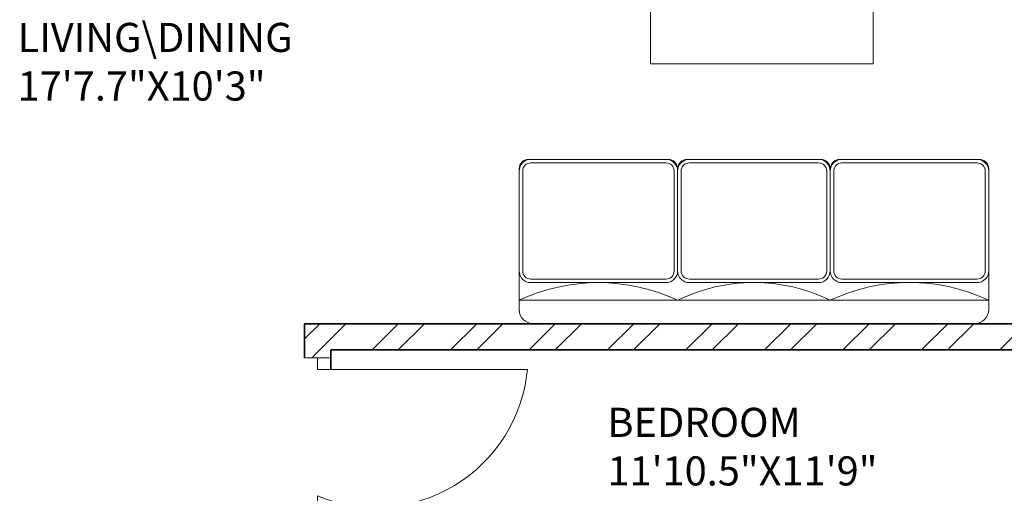
# Model space of a CAD drawing. Units: inches. Extents: x 2120 to 4013, y 1390 to 3019.
# Tile 12 of 59: x 2448 to 2617, y 1702 to 1784. Entities that reach past the tile are written whole.
import ezdxf

# ---------------------------------------------------------------- set-up
doc = ezdxf.new("R2010")
doc.units = ezdxf.units.IN
for name, color, linetype, lineweight in [('A-AREA-IDEN', 7, 'Continuous', 18), ('A-DOOR', 3, 'Continuous', 18), ('A-FURN', 8, 'Continuous', 13), ('A-WALL', 7, 'Continuous', 35), ('A-WALL-PATT', 252, 'Continuous', 13)]:
    doc.layers.add(name, color=color, linetype=linetype, lineweight=lineweight)
doc.styles.get("Standard").update_dxf_attribs({"font": 'arial.ttf'})

# ---------------------------------------------------------------- blocks, each defined once
blk = doc.blocks.new('DOOR-SWING-36IN-107p00DEG')
for p, q in [((4.5, 26.58), (0, 26.58)), ((0, 26.58), (2.25, 26.58)), ((2.25, 26.58), (2.25, 24.58)), ((2.25, 24.58), (38.25, 24.58)), ((2.25, 0), (2.25, 2.87)), ((4.5, 0), (0, 0)), ((0, 0), (2.25, 0))]:
    blk.add_line(p, q)
blk.add_arc((12.22, 27.04), 26.15, 247.599, 354.5999)
blk = doc.blocks.new('TABLE-COFFEE')
blk.add_lwpolyline([(0, 38.19), (21.88, 38.19), (21.88, 0), (0, 0)], close=True)

msp = doc.modelspace()

# ---------------------------------------------------------------- hatches: boundary and pattern name
at = {"layer": 'A-WALL-PATT'}
h = msp.add_hatch(dxfattribs=at)
h.set_pattern_fill('ANSI32', color=256)
h.paths.add_polyline_path([(2271.7331, 2343.531), (2283.3788, 2343.531), (2283.3788, 2348.031), (2283.3788, 2352.5306), (2262.7331, 2352.5306), (2262.7331, 2182.638), (2267.2331, 2182.638), (2271.7331, 2182.638), (2271.7331, 2219.031), (2391.7331, 2219.031), (2391.7331, 2214.189), (2393.9831, 2214.189), (2396.2331, 2214.189), (2396.2331, 2219.031), (2420.2331, 2219.031), (2420.2331, 2225.7535), (2417.2197, 2225.7535), (2415.7331, 2225.7535), (2415.7331, 2223.5306), (2271.7331, 2223.5306)])
h.paths.add_polyline_path([(2380.0942, 2352.5306), (2343.3788, 2352.5306), (2343.3788, 2343.531), (2363.2331, 2343.531), (2363.2331, 2288.8489), (2365.4831, 2288.8489), (2367.7331, 2288.8489), (2367.7331, 2343.531), (2380.0942, 2343.531)], flags=17)
h.paths.add_polyline_path([(2432.4339, 2352.5306), (2404.0943, 2352.5306), (2404.0943, 2343.531), (2415.7331, 2343.531), (2415.7331, 2264.0306), (2367.7331, 2264.0306), (2367.7331, 2266.4872), (2363.2331, 2266.4872), (2363.2331, 2259.531), (2367.7331, 2259.531), (2415.7331, 2259.531), (2415.7331, 2255.0658), (2420.2331, 2255.0658), (2420.2331, 2259.531), (2424.5717, 2259.531), (2424.5717, 2261.781), (2424.5717, 2264.0306), (2420.2331, 2264.0306), (2420.2331, 2343.531), (2432.4339, 2343.531)])
h.paths.add_polyline_path([(2508.9115, 2352.5306), (2456.4339, 2352.5306), (2456.4339, 2343.531), (2468.2331, 2343.531), (2468.2331, 2264.0306), (2448.0487, 2264.0306), (2448.0487, 2259.531), (2468.2331, 2259.531), (2468.2331, 2255.5496), (2472.7331, 2255.5496), (2472.7331, 2343.531), (2508.9115, 2343.531)])
h.paths.add_polyline_path([(2637.7331, 2352.5306), (2544.9116, 2352.5306), (2544.9116, 2343.531), (2589.7331, 2343.531), (2633.2331, 2343.531), (2637.7331, 2343.531)])
h.paths.add_polyline_path([(2594.2331, 2343.5306), (2589.7331, 2343.5306), (2589.7331, 2259.5306), (2589.7331, 2252.4915), (2591.9831, 2252.4915), (2594.2331, 2252.4915)])
h.paths.add_polyline_path([(2637.7331, 2223.5306), (2594.2331, 2223.5306), (2594.2331, 2230.1988), (2591.9831, 2230.1988), (2589.7331, 2230.1988), (2589.7331, 2223.5306), (2472.7331, 2223.5306), (2468.2331, 2223.5306), (2468.2331, 2219.031), (2628.7331, 2219.031), (2628.7331, 2138.031), (2637.7331, 2138.031)])
h.paths.add_polyline_path([(3822.6535, 2458.4402), (3874.9468, 2458.4402), (3874.9468, 2476.9866), (3822.6535, 2476.9866)], flags=9)
h.paths.add_polyline_path([(3834.6921, 2781.8174), (3935.9206, 2781.8174), (3935.9206, 2800.3638), (3834.6921, 2800.3638)], flags=9)
h.paths.add_polyline_path([(3832.2843, 2837.9683), (3884.5776, 2837.9683), (3884.5776, 2856.5146), (3832.2843, 2856.5146)], flags=9)
h.paths.add_polyline_path([(3830.9388, 2861.4782), (3956.8958, 2861.4782), (3956.8958, 2880.0245), (3830.9388, 2880.0245)], flags=9)
h.paths.add_polyline_path([(3870.6966, 2352.5752), (3887.9272, 2352.5752), (3887.9272, 2377.3037), (3870.6966, 2377.3037)], flags=9)
h.paths.add_polyline_path([(3289.2701, 2413.161), (3435.2223, 2413.161), (3435.2223, 2450.2538), (3289.2701, 2450.2538)], flags=9)
h.paths.add_polyline_path([(2487.6944, 2414.3601), (2637.8335, 2414.3601), (2637.8335, 2451.4528), (2487.6944, 2451.4528)], flags=9)
h.paths.add_polyline_path([(2567.3724, 1457.9199), (2815.296, 1457.9199), (2815.296, 1495.0127), (2567.3724, 1495.0127)], flags=9)
h.paths.add_polyline_path([(2655.3825, 2093.2363), (2685.9555, 2093.2363), (2685.9555, 2111.8937), (2655.3825, 2111.8937)], flags=9)
h.paths.add_polyline_path([(2543.9218, 1550.6671), (2587.8406, 1550.6671), (2587.8406, 1569.3244), (2543.9218, 1569.3244)], flags=9)
h.paths.add_polyline_path([(2905.1384, 1543.8113), (2949.0572, 1543.8113), (2949.0572, 1562.4686), (2905.1384, 1562.4686)], flags=9)
h.paths.add_polyline_path([(2736.4118, 1702.4736), (2784.2153, 1702.4736), (2784.2153, 1721.1309), (2736.4118, 1721.1309)], flags=9)
h.paths.add_polyline_path([(2912.8666, 1710.4168), (2951.707, 1710.4168), (2951.707, 1729.0741), (2912.8666, 1729.0741)], flags=9)
h.paths.add_polyline_path([(2923.5785, 1763.5038), (2959.7279, 1763.5038), (2959.7279, 1782.1611), (2923.5785, 1782.1611)], flags=9)
h.paths.add_polyline_path([(2925.2114, 1809.6137), (2967.1861, 1809.6137), (2967.1861, 1828.271), (2925.2114, 1828.271)], flags=9)
h.paths.add_polyline_path([(2996.2711, 1878.9003), (2996.2711, 1913.109), (2977.6138, 1913.109), (2977.6138, 1878.9003)], flags=9)
h.paths.add_polyline_path([(2883.0859, 1895.7192), (2927.1855, 1895.7192), (2927.1855, 1914.3766), (2883.0859, 1914.3766)], flags=9)
h.paths.add_polyline_path([(2787.3924, 1810.8013), (2841.0213, 1810.8013), (2841.0213, 1829.4587), (2787.3924, 1829.4587)], flags=9)
h.paths.add_polyline_path([(2775.6399, 2101.7395), (2829.2689, 2101.7395), (2829.2689, 2120.3968), (2775.6399, 2120.3968)], flags=9)
h.paths.add_polyline_path([(2913.0263, 2075.817), (2951.8667, 2075.817), (2951.8667, 2094.4744), (2913.0263, 2094.4744)], flags=9)
h.paths.add_polyline_path([(2929.966, 2133.3669), (2966.1154, 2133.3669), (2966.1154, 2152.0243), (2929.966, 2152.0243)], flags=9)
h.paths.add_polyline_path([(2932.7502, 2182.6088), (2968.8996, 2182.6088), (2968.8996, 2201.2662), (2932.7502, 2201.2662)], flags=9)
h.paths.add_polyline_path([(2996.0681, 2266.3173), (2996.0681, 2300.5261), (2977.4108, 2300.5261), (2977.4108, 2266.3173)], flags=9)
h.paths.add_polyline_path([(2885.1039, 2279.2186), (2929.2035, 2279.2186), (2929.2035, 2297.8759), (2885.1039, 2297.8759)], flags=9)
h.paths.add_polyline_path([(2735.7042, 2218.3197), (2783.5078, 2218.3197), (2783.5078, 2236.9771), (2735.7042, 2236.9771)], flags=9)
h.paths.add_polyline_path([(2635.6049, 2044.0085), (2648.9678, 2044.0085), (2648.9678, 2054.312), (2635.6049, 2054.312)], flags=9)
h.paths.add_polyline_path([(2714.0148, 1923.0473), (2727.3777, 1923.0473), (2727.3777, 1933.3508), (2714.0148, 1933.3508)], flags=9)
h.paths.add_polyline_path([(2709.0345, 1988.1628), (2722.3974, 1988.1628), (2722.3974, 1998.4663), (2709.0345, 1998.4663)], flags=9)
h.paths.add_polyline_path([(2592.8935, 1962.1763), (2606.2564, 1962.1763), (2606.2564, 1972.4799), (2592.8935, 1972.4799)], flags=9)
h.paths.add_polyline_path([(2618.3996, 1985.9724), (2644.1942, 1985.9724), (2644.1942, 1996.2759), (2618.3996, 1996.2759)], flags=9)
h.paths.add_polyline_path([(2601.279, 1920.5869), (2614.6419, 1920.5869), (2614.6419, 1930.8904), (2601.279, 1930.8904)], flags=9)
h.paths.add_polyline_path([(2692.3278, 1932.7645), (2704.5311, 1932.7645), (2704.5311, 1943.0681), (2692.3278, 1943.0681)], flags=9)
h.paths.add_polyline_path([(2311.122, 1672.7318), (2355.0408, 1672.7318), (2355.0408, 1691.3892), (2311.122, 1691.3892)], flags=9)
h.paths.add_polyline_path([(2456.2551, 1632.3198), (2492.4796, 1632.3198), (2492.4796, 1650.9772), (2456.2551, 1650.9772)], flags=9)
h.paths.add_polyline_path([(2401.0766, 1631.4793), (2437.301, 1631.4793), (2437.301, 1650.1367), (2401.0766, 1650.1367)], flags=9)
h.paths.add_polyline_path([(2546.7054, 1700.9235), (2594.509, 1700.9235), (2594.509, 1719.5809), (2546.7054, 1719.5809)], flags=9)
h.paths.add_polyline_path([(2445.4866, 1766.9937), (2497.5261, 1766.9937), (2497.5261, 1785.651), (2445.4866, 1785.651)], flags=9)
h.paths.add_polyline_path([(2287.9992, 1739.7675), (2326.8396, 1739.7675), (2326.8396, 1758.4248), (2287.9992, 1758.4248)], flags=9)
h.paths.add_polyline_path([(2458.5279, 1924.7607), (2510.5675, 1924.7607), (2510.5675, 1943.4181), (2458.5279, 1943.4181)], flags=9)
h.paths.add_polyline_path([(2309.2811, 1902.7642), (2345.4305, 1902.7642), (2345.4305, 1921.4215), (2309.2811, 1921.4215)], flags=9)
h.paths.add_polyline_path([(2490.7554, 2018.9392), (2530.7896, 2018.9392), (2530.7896, 2037.5965), (2490.7554, 2037.5965)], flags=9)
h.paths.add_polyline_path([(2402.143, 2024.7393), (2438.5414, 2024.7393), (2438.5414, 2043.3966), (2402.143, 2043.3966)], flags=9)
h.paths.add_polyline_path([(2287.856, 1931.7926), (2326.6964, 1931.7926), (2326.6964, 1950.4499), (2287.856, 1950.4499)], flags=9)
h.paths.add_polyline_path([(2281.7979, 2193.5771), (2320.6383, 2193.5771), (2320.6383, 2212.2344), (2281.7979, 2212.2344)], flags=25)
h.paths.add_polyline_path([(2484.0754, 2093.892), (2536.115, 2093.892), (2536.115, 2112.5494), (2484.0754, 2112.5494)], flags=9)
h.paths.add_polyline_path([(2624.7948, 2281.8639), (2624.7948, 2311.4137), (2606.1375, 2311.4137), (2606.1375, 2281.8639)], flags=9)
h.paths.add_polyline_path([(2507.5036, 2290.3639), (2541.934, 2290.3639), (2541.934, 2309.0212), (2507.5036, 2309.0212)], flags=9)
h.paths.add_polyline_path([(2423.1076, 2285.2202), (2459.332, 2285.2202), (2459.332, 2303.8776), (2423.1076, 2303.8776)], flags=9)
h.paths.add_polyline_path([(2374.5467, 2289.6272), (2410.7711, 2289.6272), (2410.7711, 2308.2846), (2374.5467, 2308.2846)], flags=25)
h.paths.add_polyline_path([(2277.4907, 2227.5651), (2316.3311, 2227.5651), (2316.3311, 2246.2224), (2277.4907, 2246.2224)], flags=25)
h.paths.add_polyline_path([(2655.3825, 2093.2367), (2685.9555, 2093.2367), (2685.9555, 2111.894), (2655.3825, 2111.894)], flags=9)
h.paths.add_polyline_path([(2543.9217, 1550.6674), (2587.8406, 1550.6674), (2587.8406, 1569.3247), (2543.9217, 1569.3247)], flags=9)
h.paths.add_polyline_path([(2905.1384, 1543.8116), (2949.0572, 1543.8116), (2949.0572, 1562.4689), (2905.1384, 1562.4689)], flags=9)
h.paths.add_polyline_path([(2736.4118, 1702.4739), (2784.2153, 1702.4739), (2784.2153, 1721.1312), (2736.4118, 1721.1312)], flags=9)
h.paths.add_polyline_path([(2912.8666, 1710.4171), (2951.707, 1710.4171), (2951.707, 1729.0744), (2912.8666, 1729.0744)], flags=9)
h.paths.add_polyline_path([(2923.5785, 1763.5041), (2959.7279, 1763.5041), (2959.7279, 1782.1614), (2923.5785, 1782.1614)], flags=9)
h.paths.add_polyline_path([(2925.2114, 1809.614), (2967.1861, 1809.614), (2967.1861, 1828.2713), (2925.2114, 1828.2713)], flags=9)
h.paths.add_polyline_path([(2996.2711, 1878.9006), (2996.2711, 1913.1094), (2977.6137, 1913.1094), (2977.6137, 1878.9006)], flags=9)
h.paths.add_polyline_path([(2883.0859, 1895.7195), (2927.1855, 1895.7195), (2927.1855, 1914.3769), (2883.0859, 1914.3769)], flags=9)
h.paths.add_polyline_path([(2787.3924, 1810.8016), (2841.0213, 1810.8016), (2841.0213, 1829.459), (2787.3924, 1829.459)], flags=9)
h.paths.add_polyline_path([(2775.6399, 2101.7398), (2829.2688, 2101.7398), (2829.2688, 2120.3971), (2775.6399, 2120.3971)], flags=9)
h.paths.add_polyline_path([(2913.0263, 2075.8173), (2951.8667, 2075.8173), (2951.8667, 2094.4747), (2913.0263, 2094.4747)], flags=9)
h.paths.add_polyline_path([(2929.966, 2133.3672), (2966.1154, 2133.3672), (2966.1154, 2152.0246), (2929.966, 2152.0246)], flags=9)
h.paths.add_polyline_path([(2932.7502, 2182.6091), (2968.8996, 2182.6091), (2968.8996, 2201.2665), (2932.7502, 2201.2665)], flags=9)
h.paths.add_polyline_path([(2996.0681, 2266.3176), (2996.0681, 2300.5264), (2977.4108, 2300.5264), (2977.4108, 2266.3176)], flags=9)
h.paths.add_polyline_path([(2885.1039, 2279.2189), (2929.2035, 2279.2189), (2929.2035, 2297.8762), (2885.1039, 2297.8762)], flags=9)
h.paths.add_polyline_path([(2735.7042, 2218.32), (2783.5078, 2218.32), (2783.5078, 2236.9774), (2735.7042, 2236.9774)], flags=9)
h.paths.add_polyline_path([(2635.6048, 2044.0088), (2648.9677, 2044.0088), (2648.9677, 2054.3123), (2635.6048, 2054.3123)], flags=9)
h.paths.add_polyline_path([(2714.0148, 1923.0476), (2727.3777, 1923.0476), (2727.3777, 1933.3511), (2714.0148, 1933.3511)], flags=9)
h.paths.add_polyline_path([(2709.0345, 1988.1631), (2722.3974, 1988.1631), (2722.3974, 1998.4666), (2709.0345, 1998.4666)], flags=9)
h.paths.add_polyline_path([(2592.8935, 1962.1766), (2606.2564, 1962.1766), (2606.2564, 1972.4802), (2592.8935, 1972.4802)], flags=9)
h.paths.add_polyline_path([(2618.3995, 1985.9727), (2644.1942, 1985.9727), (2644.1942, 1996.2762), (2618.3995, 1996.2762)], flags=9)
h.paths.add_polyline_path([(2601.279, 1920.5872), (2614.6419, 1920.5872), (2614.6419, 1930.8908), (2601.279, 1930.8908)], flags=9)
h.paths.add_polyline_path([(2692.3278, 1932.7648), (2704.5311, 1932.7648), (2704.5311, 1943.0684), (2692.3278, 1943.0684)], flags=9)
h.paths.add_polyline_path([(2311.122, 1672.7321), (2355.0408, 1672.7321), (2355.0408, 1691.3895), (2311.122, 1691.3895)], flags=9)
h.paths.add_polyline_path([(2456.2551, 1632.3201), (2492.4795, 1632.3201), (2492.4795, 1650.9775), (2456.2551, 1650.9775)], flags=9)
h.paths.add_polyline_path([(2401.0766, 1631.4796), (2437.301, 1631.4796), (2437.301, 1650.137), (2401.0766, 1650.137)], flags=9)
h.paths.add_polyline_path([(2546.7054, 1700.9238), (2594.509, 1700.9238), (2594.509, 1719.5812), (2546.7054, 1719.5812)], flags=9)
h.paths.add_polyline_path([(2445.4866, 1766.994), (2497.5261, 1766.994), (2497.5261, 1785.6513), (2445.4866, 1785.6513)], flags=9)
h.paths.add_polyline_path([(2287.9992, 1739.7678), (2326.8396, 1739.7678), (2326.8396, 1758.4251), (2287.9992, 1758.4251)], flags=9)
h.paths.add_polyline_path([(2458.5279, 1924.7611), (2510.5675, 1924.7611), (2510.5675, 1943.4184), (2458.5279, 1943.4184)], flags=9)
h.paths.add_polyline_path([(2309.2811, 1902.7645), (2345.4305, 1902.7645), (2345.4305, 1921.4218), (2309.2811, 1921.4218)], flags=9)
h.paths.add_polyline_path([(2490.7554, 2018.9395), (2530.7895, 2018.9395), (2530.7895, 2037.5968), (2490.7554, 2037.5968)], flags=9)
h.paths.add_polyline_path([(2402.143, 2024.7396), (2438.5413, 2024.7396), (2438.5413, 2043.3969), (2402.143, 2043.3969)], flags=9)
h.paths.add_polyline_path([(2287.856, 1931.7929), (2326.6964, 1931.7929), (2326.6964, 1950.4502), (2287.856, 1950.4502)], flags=9)
h.paths.add_polyline_path([(2281.7979, 2193.5774), (2320.6383, 2193.5774), (2320.6383, 2212.2347), (2281.7979, 2212.2347)], flags=25)
h.paths.add_polyline_path([(2484.0754, 2093.8924), (2536.115, 2093.8924), (2536.115, 2112.5497), (2484.0754, 2112.5497)], flags=9)
h.paths.add_polyline_path([(2624.7948, 2281.8642), (2624.7948, 2311.414), (2606.1374, 2311.414), (2606.1374, 2281.8642)], flags=9)
h.paths.add_polyline_path([(2507.5035, 2290.3642), (2541.934, 2290.3642), (2541.934, 2309.0215), (2507.5035, 2309.0215)], flags=9)
h.paths.add_polyline_path([(2423.1075, 2285.2205), (2459.332, 2285.2205), (2459.332, 2303.8779), (2423.1075, 2303.8779)], flags=9)
h.paths.add_polyline_path([(2374.5467, 2289.6275), (2410.7711, 2289.6275), (2410.7711, 2308.2849), (2374.5467, 2308.2849)], flags=25)
h.paths.add_polyline_path([(2277.4907, 2227.5654), (2316.3311, 2227.5654), (2316.3311, 2246.2227), (2277.4907, 2246.2227)], flags=25)
h = msp.add_hatch(dxfattribs=at)
h.set_pattern_fill('ANSI32', color=256)
h.paths.add_polyline_path([(2271.7331, 1980.389), (2262.7331, 1980.389), (2262.7331, 1912.8434), (2267.2331, 1912.8434), (2271.7331, 1912.8434), (2271.7331, 1922.531), (2351.2331, 1922.531), (2351.2331, 1901.4728), (2355.7331, 1901.4728), (2355.7331, 1922.531), (2357.9815, 1922.531), (2357.9815, 1926.5306), (2271.7331, 1926.5306)])
h.paths.add_polyline_path([(2589.2331, 1949.1622), (2584.7331, 1949.1622), (2580.2331, 1949.1622), (2580.2331, 1874.5306), (2355.7331, 1874.5306), (2355.7331, 1880.1922), (2351.2331, 1880.1922), (2351.2331, 1874.5306), (2271.7331, 1874.5306), (2271.7331, 1888.8431), (2262.7331, 1888.8431), (2262.7331, 1842.2909), (2267.2331, 1842.2909), (2271.7331, 1842.2909), (2271.7331, 1865.531), (2415.7331, 1865.531), (2415.7331, 1779.7286), (2420.2331, 1779.7286), (2420.2331, 1865.531), (2589.2331, 1865.531)])
h.paths.add_polyline_path([(2271.7331, 1782.2906), (2262.7331, 1782.2906), (2262.7331, 1711.4639), (2267.2331, 1711.4639), (2271.7331, 1711.4639), (2271.7331, 1738.031), (2420.2331, 1738.031), (2420.2331, 1742.531), (2420.2331, 1747.3376), (2417.9831, 1747.3376), (2415.7331, 1747.3376), (2415.7331, 1742.5306), (2271.7331, 1742.5306)])
h.paths.add_polyline_path([(2271.7331, 1627.031), (2362.3957, 1627.031), (2362.3957, 1629.281), (2362.3957, 1631.5306), (2271.7331, 1631.5306), (2271.7331, 1675.4636), (2262.7331, 1675.4636), (2262.7331, 1581.531), (2405.3032, 1581.531), (2405.3032, 1586.031), (2405.3032, 1590.5306), (2396.2331, 1590.5306), (2396.2331, 1691.4513), (2418.7206, 1691.4513), (2418.7206, 1695.951), (2396.2331, 1695.951), (2391.7331, 1695.951), (2391.7331, 1631.5306), (2386.7425, 1631.5306), (2386.7425, 1629.2806), (2386.7425, 1627.031), (2391.7331, 1627.031), (2391.7331, 1586.1709), (2271.7331, 1586.1709)])
h.paths.add_polyline_path([(2459.6703, 1590.5306), (2429.3032, 1590.5306), (2429.3032, 1581.531), (2459.6703, 1581.531), (2459.6703, 1586.031)])
h.paths.add_polyline_path([(2501.2331, 1590.531), (2501.2331, 1665.0195), (2498.9831, 1665.0195), (2496.7331, 1665.0195), (2496.7331, 1590.5306), (2483.8201, 1590.5306), (2483.8201, 1590.1579), (2483.6704, 1590.1579), (2483.6704, 1581.531), (2505.0196, 1581.531), (2505.0196, 1583.781), (2505.0196, 1586.0306), (2501.2331, 1586.0306)])
h.paths.add_polyline_path([(2544.1361, 1583.781), (2544.1361, 1586.0306), (2527.1368, 1586.0306), (2527.1368, 1583.7806), (2527.1368, 1581.531), (2544.1361, 1581.531)])
h.paths.add_polyline_path([(3822.6535, 2458.4402), (3874.9468, 2458.4402), (3874.9468, 2476.9866), (3822.6535, 2476.9866)], flags=9)
h.paths.add_polyline_path([(3834.6921, 2781.8174), (3935.9206, 2781.8174), (3935.9206, 2800.3638), (3834.6921, 2800.3638)], flags=9)
h.paths.add_polyline_path([(3832.2843, 2837.9683), (3884.5776, 2837.9683), (3884.5776, 2856.5146), (3832.2843, 2856.5146)], flags=9)
h.paths.add_polyline_path([(3830.9388, 2861.4782), (3956.8958, 2861.4782), (3956.8958, 2880.0245), (3830.9388, 2880.0245)], flags=9)
h.paths.add_polyline_path([(3870.6966, 2352.5752), (3887.9272, 2352.5752), (3887.9272, 2377.3037), (3870.6966, 2377.3037)], flags=9)
h.paths.add_polyline_path([(3289.2701, 2413.161), (3435.2223, 2413.161), (3435.2223, 2450.2538), (3289.2701, 2450.2538)], flags=9)
h.paths.add_polyline_path([(2487.6944, 2414.3601), (2637.8335, 2414.3601), (2637.8335, 2451.4528), (2487.6944, 2451.4528)], flags=9)
h.paths.add_polyline_path([(2567.3724, 1457.9199), (2815.296, 1457.9199), (2815.296, 1495.0127), (2567.3724, 1495.0127)], flags=9)
h.paths.add_polyline_path([(2655.3825, 2093.2363), (2685.9555, 2093.2363), (2685.9555, 2111.8937), (2655.3825, 2111.8937)], flags=9)
h.paths.add_polyline_path([(2543.9218, 1550.6671), (2587.8406, 1550.6671), (2587.8406, 1569.3244), (2543.9218, 1569.3244)], flags=9)
h.paths.add_polyline_path([(2905.1384, 1543.8113), (2949.0572, 1543.8113), (2949.0572, 1562.4686), (2905.1384, 1562.4686)], flags=9)
h.paths.add_polyline_path([(2736.4118, 1702.4736), (2784.2153, 1702.4736), (2784.2153, 1721.1309), (2736.4118, 1721.1309)], flags=9)
h.paths.add_polyline_path([(2912.8666, 1710.4168), (2951.707, 1710.4168), (2951.707, 1729.0741), (2912.8666, 1729.0741)], flags=9)
h.paths.add_polyline_path([(2923.5785, 1763.5038), (2959.7279, 1763.5038), (2959.7279, 1782.1611), (2923.5785, 1782.1611)], flags=9)
h.paths.add_polyline_path([(2925.2114, 1809.6137), (2967.1861, 1809.6137), (2967.1861, 1828.271), (2925.2114, 1828.271)], flags=9)
h.paths.add_polyline_path([(2996.2711, 1878.9003), (2996.2711, 1913.109), (2977.6138, 1913.109), (2977.6138, 1878.9003)], flags=9)
h.paths.add_polyline_path([(2883.0859, 1895.7192), (2927.1855, 1895.7192), (2927.1855, 1914.3766), (2883.0859, 1914.3766)], flags=9)
h.paths.add_polyline_path([(2787.3924, 1810.8013), (2841.0213, 1810.8013), (2841.0213, 1829.4587), (2787.3924, 1829.4587)], flags=9)
h.paths.add_polyline_path([(2775.6399, 2101.7395), (2829.2689, 2101.7395), (2829.2689, 2120.3968), (2775.6399, 2120.3968)], flags=9)
h.paths.add_polyline_path([(2913.0263, 2075.817), (2951.8667, 2075.817), (2951.8667, 2094.4744), (2913.0263, 2094.4744)], flags=9)
h.paths.add_polyline_path([(2929.966, 2133.3669), (2966.1154, 2133.3669), (2966.1154, 2152.0243), (2929.966, 2152.0243)], flags=9)
h.paths.add_polyline_path([(2932.7502, 2182.6088), (2968.8996, 2182.6088), (2968.8996, 2201.2662), (2932.7502, 2201.2662)], flags=9)
h.paths.add_polyline_path([(2996.0681, 2266.3173), (2996.0681, 2300.5261), (2977.4108, 2300.5261), (2977.4108, 2266.3173)], flags=9)
h.paths.add_polyline_path([(2885.1039, 2279.2186), (2929.2035, 2279.2186), (2929.2035, 2297.8759), (2885.1039, 2297.8759)], flags=9)
h.paths.add_polyline_path([(2735.7042, 2218.3197), (2783.5078, 2218.3197), (2783.5078, 2236.9771), (2735.7042, 2236.9771)], flags=9)
h.paths.add_polyline_path([(2635.6049, 2044.0085), (2648.9678, 2044.0085), (2648.9678, 2054.312), (2635.6049, 2054.312)], flags=9)
h.paths.add_polyline_path([(2714.0148, 1923.0473), (2727.3777, 1923.0473), (2727.3777, 1933.3508), (2714.0148, 1933.3508)], flags=9)
h.paths.add_polyline_path([(2709.0345, 1988.1628), (2722.3974, 1988.1628), (2722.3974, 1998.4663), (2709.0345, 1998.4663)], flags=9)
h.paths.add_polyline_path([(2592.8935, 1962.1763), (2606.2564, 1962.1763), (2606.2564, 1972.4799), (2592.8935, 1972.4799)], flags=9)
h.paths.add_polyline_path([(2618.3996, 1985.9724), (2644.1942, 1985.9724), (2644.1942, 1996.2759), (2618.3996, 1996.2759)], flags=9)
h.paths.add_polyline_path([(2601.279, 1920.5869), (2614.6419, 1920.5869), (2614.6419, 1930.8904), (2601.279, 1930.8904)], flags=9)
h.paths.add_polyline_path([(2692.3278, 1932.7645), (2704.5311, 1932.7645), (2704.5311, 1943.0681), (2692.3278, 1943.0681)], flags=9)
h.paths.add_polyline_path([(2311.122, 1672.7318), (2355.0408, 1672.7318), (2355.0408, 1691.3892), (2311.122, 1691.3892)], flags=25)
h.paths.add_polyline_path([(2456.2551, 1632.3198), (2492.4796, 1632.3198), (2492.4796, 1650.9772), (2456.2551, 1650.9772)], flags=9)
h.paths.add_polyline_path([(2401.0766, 1631.4793), (2437.301, 1631.4793), (2437.301, 1650.1367), (2401.0766, 1650.1367)], flags=9)
h.paths.add_polyline_path([(2546.7054, 1700.9235), (2594.509, 1700.9235), (2594.509, 1719.5809), (2546.7054, 1719.5809)], flags=9)
h.paths.add_polyline_path([(2445.4866, 1766.9937), (2497.5261, 1766.9937), (2497.5261, 1785.651), (2445.4866, 1785.651)], flags=9)
h.paths.add_polyline_path([(2287.9992, 1739.7675), (2326.8396, 1739.7675), (2326.8396, 1758.4248), (2287.9992, 1758.4248)], flags=24)
h.paths.add_polyline_path([(2458.5279, 1924.7607), (2510.5675, 1924.7607), (2510.5675, 1943.4181), (2458.5279, 1943.4181)], flags=25)
h.paths.add_polyline_path([(2309.2811, 1902.7642), (2345.4305, 1902.7642), (2345.4305, 1921.4215), (2309.2811, 1921.4215)], flags=25)
h.paths.add_polyline_path([(2490.7554, 2018.9392), (2530.7896, 2018.9392), (2530.7896, 2037.5965), (2490.7554, 2037.5965)], flags=9)
h.paths.add_polyline_path([(2402.143, 2024.7393), (2438.5414, 2024.7393), (2438.5414, 2043.3966), (2402.143, 2043.3966)], flags=9)
h.paths.add_polyline_path([(2287.856, 1931.7926), (2326.6964, 1931.7926), (2326.6964, 1950.4499), (2287.856, 1950.4499)], flags=25)
h.paths.add_polyline_path([(2281.7979, 2193.5771), (2320.6383, 2193.5771), (2320.6383, 2212.2344), (2281.7979, 2212.2344)], flags=9)
h.paths.add_polyline_path([(2484.0754, 2093.892), (2536.115, 2093.892), (2536.115, 2112.5494), (2484.0754, 2112.5494)], flags=9)
h.paths.add_polyline_path([(2624.7948, 2281.8639), (2624.7948, 2311.4137), (2606.1375, 2311.4137), (2606.1375, 2281.8639)], flags=9)
h.paths.add_polyline_path([(2507.5036, 2290.3639), (2541.934, 2290.3639), (2541.934, 2309.0212), (2507.5036, 2309.0212)], flags=9)
h.paths.add_polyline_path([(2423.1076, 2285.2202), (2459.332, 2285.2202), (2459.332, 2303.8776), (2423.1076, 2303.8776)], flags=9)
h.paths.add_polyline_path([(2374.5467, 2289.6272), (2410.7711, 2289.6272), (2410.7711, 2308.2846), (2374.5467, 2308.2846)], flags=9)
h.paths.add_polyline_path([(2277.4907, 2227.5651), (2316.3311, 2227.5651), (2316.3311, 2246.2224), (2277.4907, 2246.2224)], flags=9)
h.paths.add_polyline_path([(2655.3825, 2093.2367), (2685.9555, 2093.2367), (2685.9555, 2111.894), (2655.3825, 2111.894)], flags=9)
h.paths.add_polyline_path([(2543.9217, 1550.6674), (2587.8406, 1550.6674), (2587.8406, 1569.3247), (2543.9217, 1569.3247)], flags=9)
h.paths.add_polyline_path([(2905.1384, 1543.8116), (2949.0572, 1543.8116), (2949.0572, 1562.4689), (2905.1384, 1562.4689)], flags=9)
h.paths.add_polyline_path([(2736.4118, 1702.4739), (2784.2153, 1702.4739), (2784.2153, 1721.1312), (2736.4118, 1721.1312)], flags=9)
h.paths.add_polyline_path([(2912.8666, 1710.4171), (2951.707, 1710.4171), (2951.707, 1729.0744), (2912.8666, 1729.0744)], flags=9)
h.paths.add_polyline_path([(2923.5785, 1763.5041), (2959.7279, 1763.5041), (2959.7279, 1782.1614), (2923.5785, 1782.1614)], flags=9)
h.paths.add_polyline_path([(2925.2114, 1809.614), (2967.1861, 1809.614), (2967.1861, 1828.2713), (2925.2114, 1828.2713)], flags=9)
h.paths.add_polyline_path([(2996.2711, 1878.9006), (2996.2711, 1913.1094), (2977.6137, 1913.1094), (2977.6137, 1878.9006)], flags=9)
h.paths.add_polyline_path([(2883.0859, 1895.7195), (2927.1855, 1895.7195), (2927.1855, 1914.3769), (2883.0859, 1914.3769)], flags=9)
h.paths.add_polyline_path([(2787.3924, 1810.8016), (2841.0213, 1810.8016), (2841.0213, 1829.459), (2787.3924, 1829.459)], flags=9)
h.paths.add_polyline_path([(2775.6399, 2101.7398), (2829.2688, 2101.7398), (2829.2688, 2120.3971), (2775.6399, 2120.3971)], flags=9)
h.paths.add_polyline_path([(2913.0263, 2075.8173), (2951.8667, 2075.8173), (2951.8667, 2094.4747), (2913.0263, 2094.4747)], flags=9)
h.paths.add_polyline_path([(2929.966, 2133.3672), (2966.1154, 2133.3672), (2966.1154, 2152.0246), (2929.966, 2152.0246)], flags=9)
h.paths.add_polyline_path([(2932.7502, 2182.6091), (2968.8996, 2182.6091), (2968.8996, 2201.2665), (2932.7502, 2201.2665)], flags=9)
h.paths.add_polyline_path([(2996.0681, 2266.3176), (2996.0681, 2300.5264), (2977.4108, 2300.5264), (2977.4108, 2266.3176)], flags=9)
h.paths.add_polyline_path([(2885.1039, 2279.2189), (2929.2035, 2279.2189), (2929.2035, 2297.8762), (2885.1039, 2297.8762)], flags=9)
h.paths.add_polyline_path([(2735.7042, 2218.32), (2783.5078, 2218.32), (2783.5078, 2236.9774), (2735.7042, 2236.9774)], flags=9)
h.paths.add_polyline_path([(2635.6048, 2044.0088), (2648.9677, 2044.0088), (2648.9677, 2054.3123), (2635.6048, 2054.3123)], flags=9)
h.paths.add_polyline_path([(2714.0148, 1923.0476), (2727.3777, 1923.0476), (2727.3777, 1933.3511), (2714.0148, 1933.3511)], flags=9)
h.paths.add_polyline_path([(2709.0345, 1988.1631), (2722.3974, 1988.1631), (2722.3974, 1998.4666), (2709.0345, 1998.4666)], flags=9)
h.paths.add_polyline_path([(2592.8935, 1962.1766), (2606.2564, 1962.1766), (2606.2564, 1972.4802), (2592.8935, 1972.4802)], flags=9)
h.paths.add_polyline_path([(2618.3995, 1985.9727), (2644.1942, 1985.9727), (2644.1942, 1996.2762), (2618.3995, 1996.2762)], flags=9)
h.paths.add_polyline_path([(2601.279, 1920.5872), (2614.6419, 1920.5872), (2614.6419, 1930.8908), (2601.279, 1930.8908)], flags=9)
h.paths.add_polyline_path([(2692.3278, 1932.7648), (2704.5311, 1932.7648), (2704.5311, 1943.0684), (2692.3278, 1943.0684)], flags=9)
h.paths.add_polyline_path([(2311.122, 1672.7321), (2355.0408, 1672.7321), (2355.0408, 1691.3895), (2311.122, 1691.3895)], flags=25)
h.paths.add_polyline_path([(2456.2551, 1632.3201), (2492.4795, 1632.3201), (2492.4795, 1650.9775), (2456.2551, 1650.9775)], flags=9)
h.paths.add_polyline_path([(2401.0766, 1631.4796), (2437.301, 1631.4796), (2437.301, 1650.137), (2401.0766, 1650.137)], flags=9)
h.paths.add_polyline_path([(2546.7054, 1700.9238), (2594.509, 1700.9238), (2594.509, 1719.5812), (2546.7054, 1719.5812)], flags=9)
h.paths.add_polyline_path([(2445.4866, 1766.994), (2497.5261, 1766.994), (2497.5261, 1785.6513), (2445.4866, 1785.6513)], flags=9)
h.paths.add_polyline_path([(2287.9992, 1739.7678), (2326.8396, 1739.7678), (2326.8396, 1758.4251), (2287.9992, 1758.4251)], flags=24)
h.paths.add_polyline_path([(2458.5279, 1924.7611), (2510.5675, 1924.7611), (2510.5675, 1943.4184), (2458.5279, 1943.4184)], flags=25)
h.paths.add_polyline_path([(2309.2811, 1902.7645), (2345.4305, 1902.7645), (2345.4305, 1921.4218), (2309.2811, 1921.4218)], flags=25)
h.paths.add_polyline_path([(2490.7554, 2018.9395), (2530.7895, 2018.9395), (2530.7895, 2037.5968), (2490.7554, 2037.5968)], flags=9)
h.paths.add_polyline_path([(2402.143, 2024.7396), (2438.5413, 2024.7396), (2438.5413, 2043.3969), (2402.143, 2043.3969)], flags=9)
h.paths.add_polyline_path([(2287.856, 1931.7929), (2326.6964, 1931.7929), (2326.6964, 1950.4502), (2287.856, 1950.4502)], flags=25)
h.paths.add_polyline_path([(2281.7979, 2193.5774), (2320.6383, 2193.5774), (2320.6383, 2212.2347), (2281.7979, 2212.2347)], flags=9)
h.paths.add_polyline_path([(2484.0754, 2093.8924), (2536.115, 2093.8924), (2536.115, 2112.5497), (2484.0754, 2112.5497)], flags=9)
h.paths.add_polyline_path([(2624.7948, 2281.8642), (2624.7948, 2311.414), (2606.1374, 2311.414), (2606.1374, 2281.8642)], flags=9)
h.paths.add_polyline_path([(2507.5035, 2290.3642), (2541.934, 2290.3642), (2541.934, 2309.0215), (2507.5035, 2309.0215)], flags=9)
h.paths.add_polyline_path([(2423.1075, 2285.2205), (2459.332, 2285.2205), (2459.332, 2303.8779), (2423.1075, 2303.8779)], flags=9)
h.paths.add_polyline_path([(2374.5467, 2289.6275), (2410.7711, 2289.6275), (2410.7711, 2308.2849), (2374.5467, 2308.2849)], flags=9)
h.paths.add_polyline_path([(2277.4907, 2227.5654), (2316.3311, 2227.5654), (2316.3311, 2246.2227), (2277.4907, 2246.2227)], flags=9)
h = msp.add_hatch(dxfattribs=at)
h.set_pattern_fill('ANSI32', color=256)
h.paths.add_polyline_path([(2271.7331, 2122.6377), (2262.7331, 2122.6377), (2262.7331, 2040.3893), (2267.2331, 2040.3893), (2271.7331, 2040.3893), (2271.7331, 2044.8856), (2271.7331, 2070.531), (2391.7331, 2070.531), (2391.7331, 1926.5306), (2388.3993, 1926.5306), (2388.3993, 1922.531), (2395.7331, 1922.531), (2395.7331, 1992.531), (2400.4511, 1992.531), (2400.4511, 1997.0306), (2395.7331, 1997.0306), (2395.7331, 2070.531), (2443.7331, 2070.531), (2443.7331, 2046.1368), (2448.2331, 2046.1368), (2448.2331, 2070.531), (2580.2331, 2070.531), (2580.2331, 1997.0306), (2492.9076, 1997.0306), (2492.9076, 1992.531), (2580.2331, 1992.531), (2580.2331, 1983.9368), (2589.2331, 1983.9368), (2589.2331, 2070.531), (2589.2331, 2075.0306), (2396.2331, 2075.0306), (2396.2331, 2184.3565), (2393.9831, 2184.3565), (2391.7331, 2184.3565), (2391.7331, 2075.0306), (2271.7331, 2075.0306)])
h.paths.add_polyline_path([(2724.7331, 2138.0306), (2628.7331, 2138.0306), (2628.7331, 2070.5306), (2628.7331, 2067.0987), (2633.2331, 2067.0987), (2637.7331, 2067.0987), (2637.7331, 2070.531), (2657.3413, 2070.531), (2657.3413, 2079.5306), (2637.7331, 2079.5306), (2637.7331, 2129.031), (2715.7331, 2129.031), (2715.7331, 2079.5306), (2698.0378, 2079.5306), (2698.0378, 2070.531), (2715.7331, 2070.531), (2715.7331, 2012.1531), (2720.2331, 2012.1531), (2724.7331, 2012.1531)])
h.paths.add_polyline_path([(2724.7331, 2213.031), (2831.3209, 2213.031), (2831.3209, 2215.281), (2831.3209, 2217.5306), (2724.7331, 2217.5306), (2724.7331, 2343.531), (2751.8755, 2343.531), (2751.8755, 2352.5306), (2715.7331, 2352.5306), (2715.7331, 2138.031), (2724.7331, 2138.031)])
h.paths.add_polyline_path([(2902.53, 2352.5306), (2811.8755, 2352.5306), (2811.8755, 2343.531), (2867.2331, 2343.531), (2867.2331, 2217.5306), (2863.6364, 2217.5306), (2863.6364, 2213.031), (2871.7331, 2213.031), (2871.7331, 2217.531), (2871.7331, 2343.531), (2902.53, 2343.531)])
h.paths.add_polyline_path([(3009.7331, 2352.5306), (2938.53, 2352.5306), (2938.53, 2343.531), (2966.2331, 2343.531), (2966.2331, 2242.3281), (2968.4831, 2242.3281), (2970.7331, 2242.3281), (2970.7331, 2343.531), (3009.7331, 2343.531)])
h.paths.add_polyline_path([(3009.7331, 2217.5306), (2970.7331, 2217.5306), (2970.7331, 2220.5422), (2968.4831, 2220.5422), (2966.2331, 2220.5422), (2966.2331, 2217.5306), (2911.7752, 2217.5306), (2907.7331, 2217.5306), (2907.7331, 2213.0306), (2907.7331, 2194.9663), (2912.2331, 2194.9663), (2912.2331, 2213.031), (2970.7331, 2213.031), (3000.7331, 2213.031), (3000.7331, 2205.523), (3009.7331, 2205.523)])
h.paths.add_polyline_path([(3009.7331, 2181.5227), (3000.7331, 2181.5227), (3000.7331, 2165.0306), (2912.2331, 2165.0306), (2912.2331, 2170.8202), (2907.7331, 2170.8202), (2907.7331, 2165.0306), (2899.5169, 2165.0306), (2899.5169, 2162.7806), (2899.5169, 2160.531), (2907.7331, 2160.531), (2907.7331, 2137.3432), (2912.2331, 2137.3432), (2912.2331, 2160.531), (3000.7331, 2160.531), (3000.7331, 2150.4993), (3009.7331, 2150.4993)])
h.paths.add_polyline_path([(3009.7331, 2126.499), (3005.2331, 2126.499), (3000.7331, 2126.499), (3000.7331, 2112.5306), (2912.2331, 2112.5306), (2912.2331, 2115.6036), (2907.7331, 2115.6036), (2907.7331, 2108.031), (3000.7331, 2108.031), (3000.7331, 2084.7256), (3009.7331, 2084.7256)], flags=17)
h.paths.add_polyline_path([(3009.7331, 1971.531), (3009.7331, 2024.7253), (3000.7331, 2024.7253), (3000.7331, 2006.4153), (3000.7331, 1971.5306), (2864.2331, 1971.5306), (2864.2331, 2160.531), (2868.0522, 2160.531), (2868.0522, 2165.0306), (2859.7331, 2165.0306), (2859.7331, 1971.5306), (2724.7331, 1971.5306), (2724.7331, 1977.7012), (2715.7331, 1977.7012), (2715.7331, 1962.5306), (2715.7331, 1950.9035), (2720.2331, 1950.9035), (2724.7331, 1950.9035), (2724.7331, 1962.531), (2855.2331, 1962.531), (2859.7331, 1962.531), (2859.7331, 1835.031), (2864.2331, 1834.8158), (2864.2331, 1962.531), (2958.7331, 1962.531), (2958.7331, 1937.0925), (2963.2331, 1937.0925), (2963.2331, 1962.531), (3000.7331, 1962.531), (3009.7331, 1962.531)])
h.paths.add_polyline_path([(2724.7331, 1728.531), (2822.7164, 1728.531), (2822.7164, 1733.0306), (2724.7331, 1733.0306), (2724.7331, 1779.3416), (2715.7331, 1779.3416), (2715.7331, 1581.531), (2753.02, 1581.531), (2753.02, 1586.031), (2753.02, 1590.5306), (2724.7331, 1590.5306)])
h.paths.add_polyline_path([(2864.2331, 1590.531), (2864.2331, 1787.031), (2868.4075, 1787.031), (2868.4075, 1791.5306), (2859.7331, 1791.5306), (2859.7331, 1739.0306), (2859.7331, 1733.0306), (2854.3125, 1733.0306), (2854.3125, 1728.531), (2859.7331, 1728.531), (2859.7331, 1590.5306), (2813.02, 1590.5306), (2813.02, 1581.531), (2868.4123, 1581.531), (2868.4123, 1583.781), (2868.4123, 1586.0306), (2864.2331, 1586.0306)])
h.paths.add_polyline_path([(3009.7331, 1754.6619), (3000.7331, 1754.6619), (3000.7331, 1739.0306), (2912.2331, 1739.0306), (2912.2331, 1742.2257), (2907.7331, 1742.2257), (2907.7331, 1739.0306), (2907.7331, 1734.531), (3000.7331, 1734.531), (3000.7331, 1590.5306), (3000.7331, 1586.0306), (2971.3921, 1586.0306), (2971.3921, 1581.531), (3009.7331, 1581.531)])
h.paths.add_polyline_path([(2911.3921, 1583.781), (2911.3921, 1586.0306), (2891.2138, 1586.0306), (2891.2138, 1581.531), (2911.3921, 1581.531)])
h.paths.add_polyline_path([(3009.7331, 1799.8422), (3000.7331, 1799.8422), (3000.7331, 1791.5306), (2912.2331, 1791.5306), (2912.2331, 1796.3264), (2909.9831, 1796.3264), (2907.7331, 1796.3264), (2907.7331, 1791.5306), (2902.7033, 1791.5306), (2902.7033, 1787.031), (2907.7331, 1787.031), (2907.7331, 1761.1622), (2912.2331, 1761.1622), (2912.2331, 1787.031), (3000.7331, 1787.031), (3000.7331, 1778.6622), (3009.7331, 1778.6622)])
h.paths.add_polyline_path([(3009.7331, 1839.5306), (2963.2331, 1839.5306), (2963.2331, 1842.8629), (2960.9831, 1842.8629), (2958.7331, 1842.8629), (2958.7331, 1839.5306), (2907.7331, 1839.5306), (2907.7331, 1814.4599), (2912.2331, 1814.4599), (2912.2331, 1835.031), (3000.7331, 1835.031), (3000.7331, 1823.8425), (3009.7331, 1823.8425), (3009.7331, 1835.031)])
h.paths.add_polyline_path([(2963.2331, 1901.0922), (2960.9831, 1901.0922), (2958.7331, 1901.0922), (2958.7331, 1862.8843), (2963.2331, 1862.8843)], flags=17)
h.paths.add_polyline_path([(2724.7331, 1891.9826), (2724.7331, 1914.3416), (2715.7331, 1914.3416), (2715.7331, 1783.8416), (2637.7331, 1783.8416), (2637.7331, 1914.3416), (2628.7331, 1914.3416), (2624.7701, 1914.3416), (2624.7701, 1909.8416), (2624.7701, 1905.3419), (2628.7331, 1905.3419), (2628.7331, 1876.9915), (2628.7331, 1779.3419), (2637.7331, 1779.3419), (2715.7331, 1779.3419), (2724.7331, 1779.3419), (2724.7331, 1835.031)])
h.paths.add_polyline_path([(2637.7331, 1731.531), (2637.7331, 1779.3416), (2628.7331, 1779.3416), (2628.7331, 1731.5306), (2589.2331, 1731.5306), (2535.9814, 1731.5306), (2496.7331, 1731.5306), (2496.7331, 1725.6876), (2498.9831, 1725.6876), (2501.2331, 1725.6876), (2501.2331, 1727.031), (2628.7331, 1727.031), (2628.7331, 1680.4203), (2628.7331, 1590.5306), (2628.7331, 1586.0306), (2604.1361, 1586.0306), (2604.1361, 1581.531), (2637.7331, 1581.531), (2637.7331, 1590.531)])

# ---------------------------------------------------------------- linework, layer by layer
at = {"layer": 'A-FURN'}
for points in [[(2533.5642, 1757.7175), (2533.5642, 1740.5955, 0.41421356), (2535.5785, 1738.5812), (2558.7435, 1738.5812, 0.41421356), (2560.7579, 1740.5955), (2560.7579, 1757.7175, 0.41421356), (2558.7435, 1759.7318), (2535.5785, 1759.7318, 0.41421356)], [(2533.5642, 1757.7175), (2533.5642, 1740.5955, 0.41421356), (2535.5785, 1738.5812), (2558.7435, 1738.5812, 0.41421356), (2560.7579, 1740.5955), (2560.7579, 1757.7175, 0.41421356), (2558.7435, 1759.7318), (2535.5785, 1759.7318, 0.41421356)], [(2533.5642, 1757.7172), (2533.5642, 1740.5952, 0.41421356), (2535.5785, 1738.5809), (2558.7435, 1738.5809, 0.41421356), (2560.7579, 1740.5952), (2560.7579, 1757.7172, 0.41421356), (2558.7435, 1759.7315), (2535.5785, 1759.7315, 0.41421356)], [(2533.5642, 1757.7172), (2533.5642, 1740.5952, 0.41421356), (2535.5785, 1738.5809), (2558.7435, 1738.5809, 0.41421356), (2560.7579, 1740.5952), (2560.7579, 1757.7172, 0.41421356), (2558.7435, 1759.7315), (2535.5785, 1759.7315, 0.41421356)], [(2534.1685, 1757.7175), (2534.1685, 1740.5955, 0.41421356), (2535.5785, 1739.1855), (2558.7435, 1739.1855, 0.41421356), (2560.1536, 1740.5955), (2560.1536, 1757.7175, 0.41421356), (2558.7435, 1759.1275), (2535.5785, 1759.1275, 0.41421356)], [(2534.1685, 1757.7175), (2534.1685, 1740.5955, 0.41421356), (2535.5785, 1739.1855), (2558.7435, 1739.1855, 0.41421356), (2560.1536, 1740.5955), (2560.1536, 1757.7175, 0.41421356), (2558.7435, 1759.1275), (2535.5785, 1759.1275, 0.41421356)], [(2534.1685, 1757.7172), (2534.1685, 1740.5952, 0.41421356), (2535.5785, 1739.1852), (2558.7435, 1739.1852, 0.41421356), (2560.1536, 1740.5952), (2560.1536, 1757.7172, 0.41421356), (2558.7435, 1759.1272), (2535.5785, 1759.1272, 0.41421356)], [(2534.1685, 1757.7172), (2534.1685, 1740.5952, 0.41421356), (2535.5785, 1739.1852), (2558.7435, 1739.1852, 0.41421356), (2560.1536, 1740.5952), (2560.1536, 1757.7172, 0.41421356), (2558.7435, 1759.1272), (2535.5785, 1759.1272, 0.41421356)], [(2586.9444, 1757.7175), (2586.9444, 1740.5955, -0.41421356), (2584.93, 1738.5812), (2562.7722, 1738.5812, -0.41421356), (2560.7579, 1740.5955), (2560.7579, 1757.7175, -0.41421356), (2562.7722, 1759.7318), (2584.93, 1759.7318, -0.41421356)], [(2586.9444, 1757.7175), (2586.9444, 1740.5955, -0.41421356), (2584.93, 1738.5812), (2562.7722, 1738.5812, -0.41421356), (2560.7579, 1740.5955), (2560.7579, 1757.7175, -0.41421356), (2562.7722, 1759.7318), (2584.93, 1759.7318, -0.41421356)], [(2586.9444, 1757.7172), (2586.9444, 1740.5952, -0.41421356), (2584.9301, 1738.5809), (2562.7722, 1738.5809, -0.41421356), (2560.7579, 1740.5952), (2560.7579, 1757.7172, -0.41421356), (2562.7722, 1759.7315), (2584.9301, 1759.7315, -0.41421356)], [(2586.9444, 1757.7172), (2586.9444, 1740.5952, -0.41421356), (2584.9301, 1738.5809), (2562.7722, 1738.5809, -0.41421356), (2560.7579, 1740.5952), (2560.7579, 1757.7172, -0.41421356), (2562.7722, 1759.7315), (2584.9301, 1759.7315, -0.41421356)], [(2586.3401, 1757.7175), (2586.3401, 1740.5955, -0.41421356), (2584.93, 1739.1855), (2562.7722, 1739.1855, -0.41421356), (2561.3622, 1740.5955), (2561.3622, 1757.7175, -0.41421356), (2562.7722, 1759.1275), (2584.93, 1759.1275, -0.41421356)], [(2586.3401, 1757.7175), (2586.3401, 1740.5955, -0.41421356), (2584.93, 1739.1855), (2562.7722, 1739.1855, -0.41421356), (2561.3622, 1740.5955), (2561.3622, 1757.7175, -0.41421356), (2562.7722, 1759.1275), (2584.93, 1759.1275, -0.41421356)], [(2586.3401, 1757.7172), (2586.3401, 1740.5952, -0.41421356), (2584.9301, 1739.1852), (2562.7722, 1739.1852, -0.41421356), (2561.3622, 1740.5952), (2561.3622, 1757.7172, -0.41421356), (2562.7722, 1759.1272), (2584.9301, 1759.1272, -0.41421356)], [(2586.3401, 1757.7172), (2586.3401, 1740.5952, -0.41421356), (2584.9301, 1739.1852), (2562.7722, 1739.1852, -0.41421356), (2561.3622, 1740.5952), (2561.3622, 1757.7172, -0.41421356), (2562.7722, 1759.1272), (2584.9301, 1759.1272, -0.41421356)], [(2586.9444, 1757.7175), (2586.9444, 1740.5955, 0.41421356), (2588.9587, 1738.5812), (2612.1237, 1738.5812, 0.41421356), (2614.1381, 1740.5955), (2614.1381, 1757.7175, 0.41421356), (2612.1237, 1759.7318), (2588.9587, 1759.7318, 0.41421356)], [(2586.9444, 1757.7175), (2586.9444, 1740.5955, 0.41421356), (2588.9587, 1738.5812), (2612.1237, 1738.5812, 0.41421356), (2614.1381, 1740.5955), (2614.1381, 1757.7175, 0.41421356), (2612.1237, 1759.7318), (2588.9587, 1759.7318, 0.41421356)], [(2586.9444, 1757.7172), (2586.9444, 1740.5952, 0.41421356), (2588.9588, 1738.5809), (2612.1237, 1738.5809, 0.41421356), (2614.1381, 1740.5952), (2614.1381, 1757.7172, 0.41421356), (2612.1237, 1759.7315), (2588.9588, 1759.7315, 0.41421356)], [(2586.9444, 1757.7172), (2586.9444, 1740.5952, 0.41421356), (2588.9588, 1738.5809), (2612.1237, 1738.5809, 0.41421356), (2614.1381, 1740.5952), (2614.1381, 1757.7172, 0.41421356), (2612.1237, 1759.7315), (2588.9588, 1759.7315, 0.41421356)], [(2587.5487, 1757.7175), (2587.5487, 1740.5955, 0.41421356), (2588.9587, 1739.1855), (2612.1237, 1739.1855, 0.41421356), (2613.5338, 1740.5955), (2613.5338, 1757.7175, 0.41421356), (2612.1237, 1759.1275), (2588.9587, 1759.1275, 0.41421356)], [(2587.5487, 1757.7175), (2587.5487, 1740.5955, 0.41421356), (2588.9587, 1739.1855), (2612.1237, 1739.1855, 0.41421356), (2613.5338, 1740.5955), (2613.5338, 1757.7175, 0.41421356), (2612.1237, 1759.1275), (2588.9587, 1759.1275, 0.41421356)], [(2587.5487, 1757.7172), (2587.5487, 1740.5952, 0.41421356), (2588.9588, 1739.1852), (2612.1237, 1739.1852, 0.41421356), (2613.5338, 1740.5952), (2613.5338, 1757.7172, 0.41421356), (2612.1237, 1759.1272), (2588.9588, 1759.1272, 0.41421356)], [(2587.5487, 1757.7172), (2587.5487, 1740.5952, 0.41421356), (2588.9588, 1739.1852), (2612.1237, 1739.1852, 0.41421356), (2613.5338, 1740.5952), (2613.5338, 1757.7172, 0.41421356), (2612.1237, 1759.1272), (2588.9588, 1759.1272, 0.41421356)]]:
    msp.add_lwpolyline(points, format="xyb", close=True, dxfattribs=at)
at = {"layer": 'A-FURN', "ltscale": 0.03}
for points in [[(2559.1266, 1759.7318), (2535.1757, 1759.7318, 0.41421356), (2533.5642, 1758.1203), (2533.5642, 1733.9482, 0.41421356), (2535.9814, 1731.531), (2611.7209, 1731.531, 0.41421356), (2614.1381, 1733.9482), (2614.1381, 1758.1203, 0.41421356), (2612.5266, 1759.7318), (2588.5757, 1759.7318, 0.41421356), (2586.9642, 1758.1203, -1), (2586.9246, 1758.1203, 0.41421356), (2585.3131, 1759.7318), (2562.3892, 1759.7318, 0.41421356), (2560.7777, 1758.1203, -1), (2560.7381, 1758.1203, 0.41421356)], [(2559.1266, 1759.7318), (2535.1757, 1759.7318, 0.41421356), (2533.5642, 1758.1203), (2533.5642, 1733.9482, 0.41421356), (2535.9814, 1731.531), (2611.7209, 1731.531, 0.41421356), (2614.1381, 1733.9482), (2614.1381, 1758.1203, 0.41421356), (2612.5266, 1759.7318), (2588.5757, 1759.7318, 0.41421356), (2586.9642, 1758.1203, -1), (2586.9246, 1758.1203, 0.41421356), (2585.3131, 1759.7318), (2562.3892, 1759.7318, 0.41421356), (2560.7777, 1758.1203, -1), (2560.7381, 1758.1203, 0.41421356)], [(2559.1266, 1759.7315), (2535.1757, 1759.7315, 0.41421356), (2533.5642, 1758.12), (2533.5642, 1733.9479, 0.41421356), (2535.9814, 1731.5306), (2611.7209, 1731.5306, 0.41421356), (2614.1381, 1733.9479), (2614.1381, 1758.12, 0.41421356), (2612.5266, 1759.7315), (2588.5757, 1759.7315, 0.41421356), (2586.9642, 1758.12, -1), (2586.9246, 1758.12, 0.41421356), (2585.3131, 1759.7315), (2562.3892, 1759.7315, 0.41421356), (2560.7777, 1758.12, -1), (2560.7381, 1758.12, 0.41421356)], [(2559.1266, 1759.7315), (2535.1757, 1759.7315, 0.41421356), (2533.5642, 1758.12), (2533.5642, 1733.9479, 0.41421356), (2535.9814, 1731.5306), (2611.7209, 1731.5306, 0.41421356), (2614.1381, 1733.9479), (2614.1381, 1758.12, 0.41421356), (2612.5266, 1759.7315), (2588.5757, 1759.7315, 0.41421356), (2586.9642, 1758.12, -1), (2586.9246, 1758.12, 0.41421356), (2585.3131, 1759.7315), (2562.3892, 1759.7315, 0.41421356), (2560.7777, 1758.12, -1), (2560.7381, 1758.12, 0.41421356)]]:
    msp.add_lwpolyline(points, format="xyb", close=True, dxfattribs=at)
at = {"layer": 'A-FURN'}
for points in [[(2533.5642, 1735.5596), (2614.1381, 1735.5596)], [(2533.5642, 1735.5596), (2614.1381, 1735.5596)], [(2533.5642, 1735.5593), (2614.1381, 1735.5593)], [(2533.5642, 1735.5593), (2614.1381, 1735.5593)]]:
    msp.add_lwpolyline(points, dxfattribs=at)
for centre, radius, start, end in [((2600.5412, 1706.8552), 31.7619, 64.653824, 115.346176), ((2600.5412, 1706.8552), 31.7619, 64.653824, 115.346176), ((2600.5412, 1706.8549), 31.7619, 64.653824, 115.346176), ((2600.5412, 1706.8549), 31.7619, 64.653824, 115.346176), ((2547.161, 1706.5195), 32.0657, 64.910626, 115.089374), ((2547.161, 1706.5195), 32.0657, 64.910626, 115.089374), ((2547.161, 1706.5192), 32.0657, 64.910626, 115.089374), ((2547.161, 1706.5192), 32.0657, 64.910626, 115.089374), ((2573.8511, 1708.8695), 29.7287, 63.868999, 116.131001), ((2573.8511, 1708.8695), 29.7287, 63.868999, 116.131001), ((2573.8511, 1708.8692), 29.7287, 63.868999, 116.131001), ((2573.8511, 1708.8692), 29.7287, 63.868999, 116.131001)]:
    msp.add_arc(centre, radius, start, end, dxfattribs=at)
at = {"layer": 'A-WALL'}
for p, q in [((2496.7331, 1731.531), (2589.2331, 1731.531)), ((2496.7331, 1725.6876), (2496.7331, 1731.531)), ((2496.7331, 1725.6873), (2496.7331, 1731.5306)), ((2496.7331, 1731.5306), (2589.2331, 1731.5306)), ((2589.2331, 1731.531), (2628.7331, 1731.531)), ((2589.2331, 1731.5306), (2628.7331, 1731.5306)), ((2501.2331, 1727.031), (2628.7331, 1727.031)), ((2501.2331, 1723.6876), (2501.2331, 1727.031)), ((2501.2331, 1723.6873), (2501.2331, 1727.0306)), ((2501.2331, 1727.0306), (2628.7331, 1727.0306))]:
    msp.add_line(p, q, dxfattribs=at)

# ---------------------------------------------------------------- block references
at = {"layer": 'A-DOOR'}
for p in [(2496.7331, 1699.1039), (2496.7331, 1699.1036)]:
    msp.add_blockref('DOOR-SWING-36IN-107p00DEG', p, dxfattribs=at)
at = {"layer": 'A-FURN'}
for p, rotation in [((2594.3056, 1776.1459), 90.00000000000165), ((2594.3056, 1776.1456), 90.00000000000026)]:
    msp.add_blockref('TABLE-COFFEE', p, dxfattribs=dict(at, rotation=rotation))

# ---------------------------------------------------------------- texts
at = {"layer": 'A-AREA-IDEN', "char_height": 5, "attachment_point": 1}
for s, width, insert in [('LIVING\\\\DINING\\P17\'7.7"X10\'3"', 100.695238, (2447.4971, 1783.1633)), ('LIVING\\\\DINING\\P17\'7.7"X10\'3"', 100.695238, (2447.4971, 1783.163)), ('BEDROOM\\P11\'10.5"X11\'9"', 122.808534, (2548.716, 1717.0965)), ('BEDROOM\\P11\'10.5"X11\'9"', 122.808534, (2548.716, 1717.0962))]:
    msp.add_mtext_dynamic_manual_height_columns(s, width=width, gutter_width=12.5, heights=[0], dxfattribs=dict(at, insert=insert))

doc.saveas('drawing.dxf')
